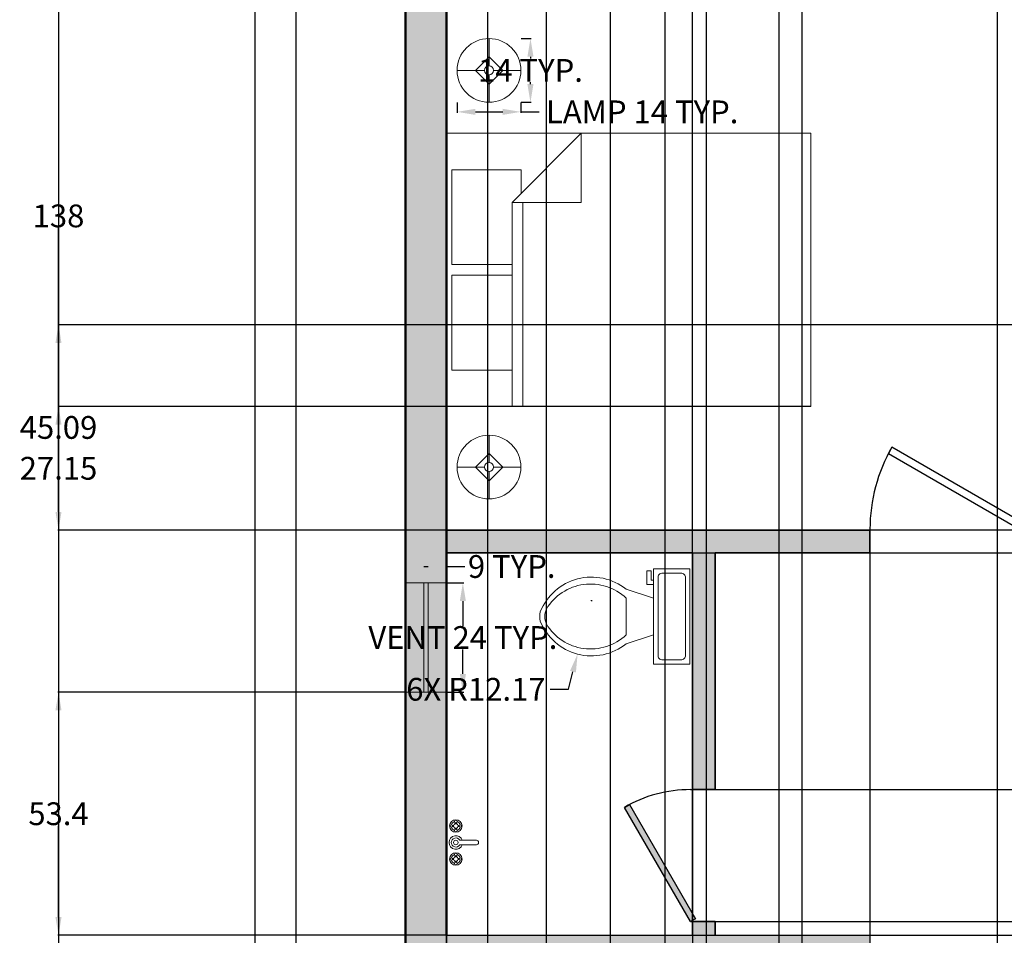
# Model space of a CAD drawing. Units: inches. Extents: x 882 to 1363, y 890 to 1847.
# Tile 7 of 9: x 898 to 1114, y 1479 to 1680. Entities that reach past the tile are written whole.
import ezdxf

# ---------------------------------------------------------------- set-up
doc = ezdxf.new("R2010")
doc.units = ezdxf.units.IN
doc.header["$MEASUREMENT"] = 0
for name, color, linetype, lineweight in [('A-ANNO-DIMS', 2, 'Continuous', 18), ('A-WALL-PATT-BNDY', 7, 'Continuous', 13), ('C-PROP', 7, 'Continuous', 25), ('doors', 3, 'Continuous', 25), ('furniture', 10, 'Continuous', 18), ('inner wall', 50, 'Continuous', 35), ('outer wall', 40, 'Continuous', 50), ('sanitary', 231, 'Continuous', 18), ('ventilator', 130, 'Continuous', 18)]:
    doc.layers.add(name, color=color, linetype=linetype, lineweight=lineweight)
doc.layers.add('A-WALL-PATT', color=251, linetype='Continuous', lineweight=13, true_color=0x636466)
doc.styles.get("Standard").update_dxf_attribs({"font": 'arial.ttf'})
doc.dimstyles.get("Standard").update_dxf_attribs({"dimtxt": 5, "dimasz": 4, "dimexe": 0.18, "dimexo": 0.0625, "dimgap": 0.09, "dimtad": 0, "dimtih": 1, "dimtoh": 1, "dimdec": 1, "dimzin": 0, "dimdsep": 46, "dimlunit": 3, "dimtxsty": 'Standard', "dimcen": 0.09, "dimadec": 0, "dimazin": 0, "dimtfac": 1, "dimtdec": 1, "dimtofl": 0, "dimtmove": 0, "dimatfit": 3, "dimfxl": 1, "dimtolj": 1, "dimtzin": 0, "dimarcsym": 0})

# ---------------------------------------------------------------- blocks, each defined once
blk = doc.blocks.new('*U3')
for p, q in [((0, 0), (0, 6)), ((40, 0), (40, 6))]:
    blk.add_line(p, q)
blk.add_lwpolyline([(0, 0), (34.64, -20), (35.52, -18.48), (0.87, 1.52)], close=True)
blk.add_arc((0, 0), 40, 330, 0)
blk = doc.blocks.new('*U5')
for p, q in [((0, 0), (0, -6)), ((40, 0), (40, -6))]:
    blk.add_line(p, q)
blk.add_lwpolyline([(0, 0), (34.64, 20), (35.52, 18.48), (0.88, -1.52)], close=True)
blk.add_arc((0, 0), 40, 0, 30)
blk = doc.blocks.new('Toilet - top')
for p, q in [((9.5, -6), (9.5, -2)), ((-10, -8.5), (-8, -8.5)), ((-10, -9.5), (-10, -8.5)), ((-8, -8.5), (-8, -8)), ((-7, -8), (-7, -9.5)), ((-4, -8), (-6, -14)), ((4, -8), (6, -14)), ((-7, -9.5), (-10, -9.5)), ((4, -14), (-4, -14))]:
    blk.add_line(p, q)
blk.add_lwpolyline([(10.5, -8), (10.5, 0), (-10.5, 0), (-10.5, -8)], close=True)
for points in [[(-9.5, -2), (-9.5, -6)], [(8.5, -1), (-8.5, -1)], [(-8.5, -7), (8.5, -7)]]:
    blk.add_lwpolyline(points)
for centre, radius, start, end in [((-8.62, -1.88), 0.884, 81.8699, 188.1301), ((8.62, -1.88), 0.884, 351.8699, 98.1301), ((-8.62, -6.12), 0.884, 171.8699, 278.1301), ((8.62, -6.12), 0.884, 261.8699, 8.1301), ((3.52, -21.58), 12.17, 141.4691, 247.9714), ((4.2, -21.82), 11.33, 136.3677, 238.9468), ((-3.52, -21.58), 12.17, 292.0284, 38.5307), ((-4.2, -21.82), 11.33, 301.053, 43.6321), ((0, -27.88), 4, 245.7318, 294.2682), ((0, -29), 4, 254.8605, 285.1395)]:
    blk.add_arc(centre, radius, start, end)
blk = doc.blocks.new('Faucet - Bathroom top')
for p, q in [((-4.107, 0.125), (-4.375, 0.125)), ((-3.75, 0.4788), (-3.75, 0.75)), ((-3.5, 0.482), (-3.5, 0.75)), ((-3.1461, 0.125), (-2.875, 0.125)), ((3.143, 0.125), (2.875, 0.125)), ((3.5, 0.4788), (3.5, 0.75)), ((3.75, 0.482), (3.75, 0.75)), ((4.1039, 0.125), (4.375, 0.125)), ((-4.1039, -0.125), (-4.375, -0.125)), ((-3.75, -0.4821), (-3.75, -0.75)), ((-3.5, -0.4789), (-3.5, -0.75)), ((-3.143, -0.125), (-2.875, -0.125)), ((-0.5, -0.8639), (-0.5, -4.5)), ((0.5, -4.5), (0.5, -0.8631)), ((3.1461, -0.125), (2.875, -0.125)), ((3.5, -0.4821), (3.5, -0.75)), ((3.75, -0.4789), (3.75, -0.75)), ((4.107, -0.125), (4.375, -0.125))]:
    blk.add_line(p, q)
for centre, radius in [((-3.625, 0), 1.375), ((-4.625, 0), 0.2795), ((-3.625, 0), 0.5), ((-3.625, 1), 0.2795), ((-2.625, 0), 0.2795), ((0, 0), 0.5), ((3.625, 0), 1.375), ((2.625, 0), 0.2795), ((3.625, 0), 0.5), ((3.625, 1), 0.2795), ((4.625, 0), 0.2795), ((-3.625, -1), 0.2795), ((3.625, -1), 0.2795)]:
    blk.add_circle(centre, radius)
for centre, radius, start, end in [((-3.625, 0), 1, 105.2407, 164.2093), ((-3.625, 0), 1, 16.44125, 74.07887), ((0, 0), 1.5, 289.6514, 250.3603), ((0, 0), 1, 300.3431, 239.7554), ((3.625, 0), 1, 106.12, 164.0884), ((3.625, 0), 1, 16.23422, 73.90469), ((-3.625, 0), 1, 196.2342, 253.9047), ((-3.625, 0), 1, 286.12, 344.0884), ((3.625, 0), 1, 196.4413, 254.0789), ((3.625, 0), 1, 285.2407, 344.2093), ((0, -4.5), 0.5, 180, 0)]:
    blk.add_arc(centre, radius, start, end)
blk = doc.blocks.new('Bed - Queen')
for p, q in [((0, -80.00003), (0, 0)), ((0, 0), (59.99999, 0)), ((59.99999, 0), (59.99999, -80.00003)), ((7.99999, -1.2), (28.79998, -1.2)), ((7.99999, -14.4), (7.99999, -1.2)), ((28.79998, -1.2), (28.79998, -14.4)), ((31.19999, -1.2), (51.99999, -1.2)), ((31.19999, -14.4), (31.19999, -1.2)), ((51.99999, -1.2), (51.99999, -16.4)), ((0, -14.4), (44.8, -14.4)), ((59.99999, -29.6), (44.8, -14.4)), ((44.8, -14.4), (44.8, -29.6)), ((44.8, -16.8), (0, -16.8)), ((51.99999, -16.4), (46.79936, -16.4)), ((44.8, -29.6), (59.99999, -29.6)), ((59.99999, -80.00003), (0, -80.00003))]:
    blk.add_line(p, q)
blk = doc.blocks.new('Lamp - Table')
for p, q in [((0, 7), (0, 1)), ((0, 3), (-3, 0)), ((3, 0), (0, 3)), ((-1, 0), (-7, 0)), ((-3, 0), (0, -3)), ((0, -3), (3, 0)), ((1, 0), (7, 0)), ((0, -1), (0, -7))]:
    blk.add_line(p, q)
for radius in [7, 1]:
    blk.add_circle((0, 0), radius)
blk = doc.blocks.new('VENT-24IN-9IN')
for p, q in [((24, 5), (0, 5)), ((24, 4), (0, 4))]:
    blk.add_line(p, q)
blk.add_lwpolyline([(0, 9), (24, 9), (24, 0), (0, 0)], close=True)
blk = doc.blocks.new('*D17')
at = {"layer": 'A-ANNO-DIMS', "color": 0, "lineweight": -2, "transparency": 16777216}
for p, q in [((994.18, 1661.64), (994.18, 1659.42)), ((1008.18, 1661.64), (1008.18, 1659.42)), ((998.18, 1659.6), (1004.18, 1659.6)), ((1008.18, 1659.6), (1012.18, 1659.6))]:
    blk.add_line(p, q, dxfattribs=at)
at = {"layer": 'A-ANNO-DIMS', "color": 0, "transparency": 16777216}
for points in [[(998.18, 1660.27), (998.18, 1658.93), (994.18, 1659.6)], [(1004.18, 1660.27), (1004.18, 1658.93), (1008.18, 1659.6)]]:
    blk.add_solid(points, dxfattribs=at)
at = {"layer": 'Defpoints', "color": 0, "transparency": 16777216}
for p in [(994.18, 1661.7), (1008.18, 1661.7), (1008.18, 1659.6)]:
    blk.add_point(p, dxfattribs=at)
at = {"layer": 'A-ANNO-DIMS', "color": 0, "transparency": 16777216, "insert": (1034.81, 1659.6), "char_height": 5, "attachment_point": 5}
blk.add_mtext('\\A1;LAMP 14 TYP.', dxfattribs=at)
blk = doc.blocks.new('*D18')
at = {"layer": 'A-ANNO-DIMS', "color": 0, "lineweight": -2, "transparency": 16777216}
for p, q in [((1008.24, 1675.7), (1010.46, 1675.7)), ((1010.28, 1671.7), (1010.28, 1671.3)), ((1010.28, 1665.7), (1010.28, 1666.1)), ((1008.24, 1661.7), (1010.46, 1661.7))]:
    blk.add_line(p, q, dxfattribs=at)
at = {"layer": 'A-ANNO-DIMS', "color": 0, "transparency": 16777216}
for points in [[(1009.61, 1671.7), (1010.95, 1671.7), (1010.28, 1675.7)], [(1009.61, 1665.7), (1010.95, 1665.7), (1010.28, 1661.7)]]:
    blk.add_solid(points, dxfattribs=at)
at = {"layer": 'Defpoints', "color": 0, "transparency": 16777216}
for p in [(1008.18, 1675.7), (1010.28, 1675.7), (1008.18, 1661.7)]:
    blk.add_point(p, dxfattribs=at)
at = {"layer": 'A-ANNO-DIMS', "color": 0, "transparency": 16777216, "insert": (1010.28, 1668.7), "char_height": 5, "attachment_point": 5}
blk.add_mtext('\\A1;14 TYP.', dxfattribs=at)
blk = doc.blocks.new('*D25')
at = {"layer": 'A-ANNO-DIMS', "color": 0, "lineweight": -2, "transparency": 16777216}
for p, q in [((991.9, 1556.15), (995.62, 1556.15)), ((995.44, 1552.15), (995.44, 1546.75)), ((995.44, 1536.15), (995.44, 1541.55)), ((991.9, 1532.15), (995.62, 1532.15))]:
    blk.add_line(p, q, dxfattribs=at)
at = {"layer": 'A-ANNO-DIMS', "color": 0, "transparency": 16777216}
for points in [[(994.77, 1552.15), (996.11, 1552.15), (995.44, 1556.15)], [(994.77, 1536.15), (996.11, 1536.15), (995.44, 1532.15)]]:
    blk.add_solid(points, dxfattribs=at)
at = {"layer": 'Defpoints', "color": 0, "transparency": 16777216}
for p in [(991.84, 1556.15), (991.84, 1532.15), (995.44, 1532.15)]:
    blk.add_point(p, dxfattribs=at)
at = {"layer": 'A-ANNO-DIMS', "color": 0, "transparency": 16777216, "insert": (995.44, 1544.15), "char_height": 5, "attachment_point": 5}
blk.add_mtext('\\A1;VENT 24 TYP.', dxfattribs=at)
blk = doc.blocks.new('*D26')
at = {"layer": 'A-ANNO-DIMS', "color": 0, "lineweight": -2, "transparency": 16777216}
for p, q in [((982.84, 1556.22), (982.84, 1559.93)), ((986.84, 1559.75), (987.84, 1559.75)), ((991.84, 1556.22), (991.84, 1559.93)), ((991.84, 1559.75), (995.84, 1559.75))]:
    blk.add_line(p, q, dxfattribs=at)
at = {"layer": 'A-ANNO-DIMS', "color": 0, "transparency": 16777216}
for points in [[(986.84, 1560.42), (986.84, 1559.09), (982.84, 1559.75)], [(987.84, 1560.42), (987.84, 1559.09), (991.84, 1559.75)]]:
    blk.add_solid(points, dxfattribs=at)
at = {"layer": 'Defpoints', "color": 0, "transparency": 16777216}
for p in [(991.84, 1559.75), (982.84, 1556.15), (991.84, 1556.15)]:
    blk.add_point(p, dxfattribs=at)
at = {"layer": 'A-ANNO-DIMS', "color": 0, "transparency": 16777216, "insert": (1006.16, 1559.75), "char_height": 5, "attachment_point": 5}
blk.add_mtext('\\A1;9 TYP.', dxfattribs=at)
blk = doc.blocks.new('*D37')
at = {"layer": 'A-ANNO-DIMS', "color": 0, "lineweight": -2, "transparency": 16777216}
for p, q in [((982.78, 1767.75), (906.46, 1767.75)), ((906.64, 1763.75), (906.64, 1383.34)), ((906.64, 997.75), (906.64, 1378.16)), ((982.78, 993.75), (906.46, 993.75))]:
    blk.add_line(p, q, dxfattribs=at)
at = {"layer": 'A-ANNO-DIMS', "color": 0, "transparency": 16777216}
for points in [[(905.97, 1763.75), (907.3, 1763.75), (906.64, 1767.75)], [(905.97, 997.75), (907.3, 997.75), (906.64, 993.75)]]:
    blk.add_solid(points, dxfattribs=at)
at = {"layer": 'Defpoints', "color": 0, "transparency": 16777216}
for p in [(906.64, 1767.75), (982.84, 1767.75), (982.84, 993.75)]:
    blk.add_point(p, dxfattribs=at)
at = {"layer": 'A-ANNO-DIMS', "color": 0, "transparency": 16777216, "insert": (906.64, 1380.75), "char_height": 5, "attachment_point": 5}
blk.add_mtext('\\A1;774', dxfattribs=at)
blk = doc.blocks.new('*D40')
at = {"layer": 'A-ANNO-DIMS', "color": 0, "lineweight": -2, "transparency": 16777216}
for p, q in [((991.84, 1758.69), (991.84, 893.37)), ((1064.84, 1758.69), (1064.84, 893.37)), ((995.84, 893.55), (1024.69, 893.55)), ((1060.84, 893.55), (1031.99, 893.55))]:
    blk.add_line(p, q, dxfattribs=at)
at = {"layer": 'A-ANNO-DIMS', "color": 0, "transparency": 16777216}
for points in [[(995.84, 894.21), (995.84, 892.88), (991.84, 893.55)], [(1060.84, 894.21), (1060.84, 892.88), (1064.84, 893.55)]]:
    blk.add_solid(points, dxfattribs=at)
at = {"layer": 'Defpoints', "color": 0, "transparency": 16777216}
for p in [(991.84, 1758.75), (1064.84, 1758.75), (1064.84, 893.55)]:
    blk.add_point(p, dxfattribs=at)
at = {"layer": 'A-ANNO-DIMS', "color": 0, "transparency": 16777216, "insert": (1028.34, 893.55), "char_height": 5, "attachment_point": 5}
blk.add_mtext('\\A1;73', dxfattribs=at)
blk = doc.blocks.new('*D41')
at = {"layer": 'A-ANNO-DIMS', "color": 0, "lineweight": -2, "transparency": 16777216}
for p, q in [((1069.84, 1758.69), (1069.84, 893.37)), ((1154.84, 1758.69), (1154.84, 893.37)), ((1073.84, 893.55), (1108.65, 893.55)), ((1150.84, 893.55), (1116.03, 893.55))]:
    blk.add_line(p, q, dxfattribs=at)
at = {"layer": 'A-ANNO-DIMS', "color": 0, "transparency": 16777216}
for points in [[(1073.84, 894.21), (1073.84, 892.88), (1069.84, 893.55)], [(1150.84, 894.21), (1150.84, 892.88), (1154.84, 893.55)]]:
    blk.add_solid(points, dxfattribs=at)
at = {"layer": 'Defpoints', "color": 0, "transparency": 16777216}
for p in [(1069.84, 1758.75), (1154.84, 1758.75), (1154.84, 893.55)]:
    blk.add_point(p, dxfattribs=at)
at = {"layer": 'A-ANNO-DIMS', "color": 0, "transparency": 16777216, "insert": (1112.34, 893.55), "char_height": 5, "attachment_point": 5}
blk.add_mtext('\\A1;85', dxfattribs=at)
blk = doc.blocks.new('*D44')
at = {"layer": 'A-ANNO-DIMS', "color": 0, "lineweight": -2, "transparency": 16777216}
for p, q in [((1243.78, 1705.75), (906.46, 1705.75)), ((906.64, 1701.75), (906.64, 1639.39)), ((906.64, 1571.75), (906.64, 1634.1)), ((1243.78, 1567.75), (906.46, 1567.75))]:
    blk.add_line(p, q, dxfattribs=at)
at = {"layer": 'A-ANNO-DIMS', "color": 0, "transparency": 16777216}
for points in [[(905.97, 1701.75), (907.3, 1701.75), (906.64, 1705.75)], [(905.97, 1571.75), (907.3, 1571.75), (906.64, 1567.75)]]:
    blk.add_solid(points, dxfattribs=at)
at = {"layer": 'Defpoints', "color": 0, "transparency": 16777216}
for p in [(1243.84, 1705.75), (906.64, 1567.75), (1243.84, 1567.75)]:
    blk.add_point(p, dxfattribs=at)
at = {"layer": 'A-ANNO-DIMS', "color": 0, "transparency": 16777216, "insert": (906.64, 1636.75), "char_height": 5, "attachment_point": 5}
blk.add_mtext('\\A1;138', dxfattribs=at)
blk = doc.blocks.new('*D46')
at = {"layer": 'A-ANNO-DIMS', "color": 0, "lineweight": -2, "transparency": 16777216}
for p, q in [((991.84, 1567.81), (991.84, 1844.13)), ((995.84, 1843.95), (1052.49, 1843.95)), ((1119.84, 1843.95), (1063.19, 1843.95)), ((1123.84, 1567.81), (1123.84, 1844.13))]:
    blk.add_line(p, q, dxfattribs=at)
at = {"layer": 'A-ANNO-DIMS', "color": 0, "transparency": 16777216}
for points in [[(995.84, 1844.62), (995.84, 1843.29), (991.84, 1843.95)], [(1119.84, 1844.62), (1119.84, 1843.29), (1123.84, 1843.95)]]:
    blk.add_solid(points, dxfattribs=at)
at = {"layer": 'Defpoints', "color": 0, "transparency": 16777216}
for p in [(1123.84, 1843.95), (991.84, 1567.75), (1123.84, 1567.75)]:
    blk.add_point(p, dxfattribs=at)
at = {"layer": 'A-ANNO-DIMS', "color": 0, "transparency": 16777216, "insert": (1057.84, 1843.95), "char_height": 5, "attachment_point": 5}
blk.add_mtext('\\A1;132', dxfattribs=at)
blk = doc.blocks.new('*D48')
at = {"layer": 'A-ANNO-DIMS', "color": 0, "lineweight": -2, "transparency": 16777216}
for p, q in [((1084.84, 1562.69), (1084.84, 893.37)), ((1120.84, 1562.69), (1120.84, 893.37)), ((1088.84, 893.55), (1099.17, 893.55)), ((1116.84, 893.55), (1106.51, 893.55))]:
    blk.add_line(p, q, dxfattribs=at)
at = {"layer": 'A-ANNO-DIMS', "color": 0, "transparency": 16777216}
for points in [[(1088.84, 894.21), (1088.84, 892.88), (1084.84, 893.55)], [(1116.84, 894.21), (1116.84, 892.88), (1120.84, 893.55)]]:
    blk.add_solid(points, dxfattribs=at)
at = {"layer": 'Defpoints', "color": 0, "transparency": 16777216}
for p in [(1084.84, 1562.75), (1120.84, 1562.75), (1120.84, 893.55)]:
    blk.add_point(p, dxfattribs=at)
at = {"layer": 'A-ANNO-DIMS', "color": 0, "transparency": 16777216, "insert": (1102.84, 893.55), "char_height": 5, "attachment_point": 5}
blk.add_mtext('\\A1;36', dxfattribs=at)
blk = doc.blocks.new('*D51')
at = {"layer": 'A-ANNO-DIMS', "color": 0, "lineweight": -2, "transparency": 16777216}
for p, q in [((982.84, 1767.69), (982.84, 893.37)), ((1000.84, 1767.69), (1000.84, 893.37)), ((986.84, 893.55), (996.84, 893.55)), ((1000.84, 893.55), (1004.84, 893.55))]:
    blk.add_line(p, q, dxfattribs=at)
at = {"layer": 'A-ANNO-DIMS', "color": 0, "transparency": 16777216}
for points in [[(986.84, 894.21), (986.84, 892.88), (982.84, 893.55)], [(996.84, 894.21), (996.84, 892.88), (1000.84, 893.55)]]:
    blk.add_solid(points, dxfattribs=at)
at = {"layer": 'Defpoints', "color": 0, "transparency": 16777216}
for p in [(982.84, 1767.75), (1000.84, 1767.75), (1000.84, 893.55)]:
    blk.add_point(p, dxfattribs=at)
at = {"layer": 'A-ANNO-DIMS', "color": 0, "transparency": 16777216, "insert": (1015.08, 893.55), "char_height": 5, "attachment_point": 5}
blk.add_mtext('\\A1;18.006', dxfattribs=at)
blk = doc.blocks.new('*D52')
at = {"layer": 'A-ANNO-DIMS', "color": 0, "lineweight": -2, "transparency": 16777216}
for p, q in [((1048.84, 1767.69), (1048.84, 893.37)), ((1118.86, 1767.69), (1118.86, 893.37)), ((1052.84, 893.55), (1075.83, 893.55)), ((1114.86, 893.55), (1091.87, 893.55))]:
    blk.add_line(p, q, dxfattribs=at)
at = {"layer": 'A-ANNO-DIMS', "color": 0, "transparency": 16777216}
for points in [[(1052.84, 894.21), (1052.84, 892.88), (1048.84, 893.55)], [(1114.86, 894.21), (1114.86, 892.88), (1118.86, 893.55)]]:
    blk.add_solid(points, dxfattribs=at)
at = {"layer": 'Defpoints', "color": 0, "transparency": 16777216}
for p in [(1048.84, 1767.75), (1118.86, 1767.75), (1118.86, 893.55)]:
    blk.add_point(p, dxfattribs=at)
at = {"layer": 'A-ANNO-DIMS', "color": 0, "transparency": 16777216, "insert": (1083.85, 893.55), "char_height": 5, "attachment_point": 5}
blk.add_mtext('\\A1;70.01', dxfattribs=at)
blk = doc.blocks.new('*D56')
at = {"layer": 'A-ANNO-DIMS', "color": 0, "lineweight": -2, "transparency": 16777216}
for p, q in [((991.9, 1562.75), (1353.22, 1562.75)), ((1353.04, 1558.75), (1353.04, 1523.39)), ((1353.04, 1482.75), (1353.04, 1518.11)), ((991.9, 1478.75), (1353.22, 1478.75))]:
    blk.add_line(p, q, dxfattribs=at)
at = {"layer": 'A-ANNO-DIMS', "color": 0, "transparency": 16777216}
for points in [[(1352.38, 1558.75), (1353.71, 1558.75), (1353.04, 1562.75)], [(1352.38, 1482.75), (1353.71, 1482.75), (1353.04, 1478.75)]]:
    blk.add_solid(points, dxfattribs=at)
at = {"layer": 'Defpoints', "color": 0, "transparency": 16777216}
for p in [(991.84, 1562.75), (991.84, 1478.75), (1353.04, 1478.75)]:
    blk.add_point(p, dxfattribs=at)
at = {"layer": 'A-ANNO-DIMS', "color": 0, "transparency": 16777216, "insert": (1353.04, 1520.75), "char_height": 5, "attachment_point": 5}
blk.add_mtext('\\A1;84', dxfattribs=at)
blk = doc.blocks.new('*D57')
at = {"layer": 'A-ANNO-DIMS', "color": 0, "lineweight": -2, "transparency": 16777216}
for p, q in [((991.84, 1478.81), (991.84, 1844.13)), ((995.84, 1843.95), (1015.18, 1843.95)), ((1041.84, 1843.95), (1022.5, 1843.95)), ((1045.84, 1478.81), (1045.84, 1844.13))]:
    blk.add_line(p, q, dxfattribs=at)
at = {"layer": 'A-ANNO-DIMS', "color": 0, "transparency": 16777216}
for points in [[(995.84, 1844.62), (995.84, 1843.29), (991.84, 1843.95)], [(1041.84, 1844.62), (1041.84, 1843.29), (1045.84, 1843.95)]]:
    blk.add_solid(points, dxfattribs=at)
at = {"layer": 'Defpoints', "color": 0, "transparency": 16777216}
for p in [(1045.84, 1843.95), (991.84, 1478.75), (1045.84, 1478.75)]:
    blk.add_point(p, dxfattribs=at)
at = {"layer": 'A-ANNO-DIMS', "color": 0, "transparency": 16777216, "insert": (1018.84, 1843.95), "char_height": 5, "attachment_point": 5}
blk.add_mtext('\\A1;54', dxfattribs=at)
blk = doc.blocks.new('*D60')
at = {"layer": 'A-ANNO-DIMS', "color": 0, "lineweight": -2, "transparency": 16777216}
for p, q in [((1050.9, 1510.75), (1353.22, 1510.75)), ((1353.04, 1506.75), (1353.04, 1498.89)), ((1353.04, 1485.75), (1353.04, 1493.61)), ((1050.9, 1481.75), (1353.22, 1481.75))]:
    blk.add_line(p, q, dxfattribs=at)
at = {"layer": 'A-ANNO-DIMS', "color": 0, "transparency": 16777216}
for points in [[(1352.38, 1506.75), (1353.71, 1506.75), (1353.04, 1510.75)], [(1352.38, 1485.75), (1353.71, 1485.75), (1353.04, 1481.75)]]:
    blk.add_solid(points, dxfattribs=at)
at = {"layer": 'Defpoints', "color": 0, "transparency": 16777216}
for p in [(1050.84, 1510.75), (1050.84, 1481.75), (1353.04, 1481.75)]:
    blk.add_point(p, dxfattribs=at)
at = {"layer": 'A-ANNO-DIMS', "color": 0, "transparency": 16777216, "insert": (1353.04, 1496.25), "char_height": 5, "attachment_point": 5}
blk.add_mtext('\\A1;29', dxfattribs=at)
blk = doc.blocks.new('*D68')
at = {"layer": 'A-ANNO-DIMS', "color": 0, "lineweight": -2, "transparency": 16777216}
for p, q in [((1027.84, 1142.81), (1027.84, 1844.13)), ((1031.84, 1843.95), (1066.65, 1843.95)), ((1108.84, 1843.95), (1074.03, 1843.95)), ((1112.84, 1142.81), (1112.84, 1844.13))]:
    blk.add_line(p, q, dxfattribs=at)
at = {"layer": 'A-ANNO-DIMS', "color": 0, "transparency": 16777216}
for points in [[(1031.84, 1844.62), (1031.84, 1843.29), (1027.84, 1843.95)], [(1108.84, 1844.62), (1108.84, 1843.29), (1112.84, 1843.95)]]:
    blk.add_solid(points, dxfattribs=at)
at = {"layer": 'Defpoints', "color": 0, "transparency": 16777216}
for p in [(1112.84, 1843.95), (1027.84, 1142.75), (1112.84, 1142.75)]:
    blk.add_point(p, dxfattribs=at)
at = {"layer": 'A-ANNO-DIMS', "color": 0, "transparency": 16777216, "insert": (1070.34, 1843.95), "char_height": 5, "attachment_point": 5}
blk.add_mtext('\\A1;85', dxfattribs=at)
blk = doc.blocks.new('*D74')
at = {"layer": 'A-ANNO-DIMS', "color": 0, "lineweight": -2, "transparency": 16777216}
for p, q in [((991.84, 1002.81), (991.84, 1844.13)), ((995.84, 1843.95), (1012.06, 1843.95)), ((1035.84, 1843.95), (1019.62, 1843.95)), ((1039.84, 1002.81), (1039.84, 1844.13))]:
    blk.add_line(p, q, dxfattribs=at)
at = {"layer": 'A-ANNO-DIMS', "color": 0, "transparency": 16777216}
for points in [[(995.84, 1844.62), (995.84, 1843.29), (991.84, 1843.95)], [(1035.84, 1844.62), (1035.84, 1843.29), (1039.84, 1843.95)]]:
    blk.add_solid(points, dxfattribs=at)
at = {"layer": 'Defpoints', "color": 0, "transparency": 16777216}
for p in [(1039.84, 1843.95), (991.84, 1002.75), (1039.84, 1002.75)]:
    blk.add_point(p, dxfattribs=at)
at = {"layer": 'A-ANNO-DIMS', "color": 0, "transparency": 16777216, "insert": (1015.84, 1843.95), "char_height": 5, "attachment_point": 5}
blk.add_mtext('\\A1;48', dxfattribs=at)
blk = doc.blocks.new('*D85')
at = {"layer": 'A-ANNO-DIMS', "color": 0, "lineweight": -2, "transparency": 16777216}
for p, q in [((1045.84, 1562.69), (1045.84, 893.37)), ((1084.84, 1562.69), (1084.84, 893.37)), ((1049.84, 893.55), (1061.66, 893.55)), ((1080.84, 893.55), (1069.01, 893.55))]:
    blk.add_line(p, q, dxfattribs=at)
at = {"layer": 'A-ANNO-DIMS', "color": 0, "transparency": 16777216}
for points in [[(1049.84, 894.21), (1049.84, 892.88), (1045.84, 893.55)], [(1080.84, 894.21), (1080.84, 892.88), (1084.84, 893.55)]]:
    blk.add_solid(points, dxfattribs=at)
at = {"layer": 'Defpoints', "color": 0, "transparency": 16777216}
for p in [(1045.84, 1562.75), (1084.84, 1562.75), (1084.84, 893.55)]:
    blk.add_point(p, dxfattribs=at)
at = {"layer": 'A-ANNO-DIMS', "color": 0, "transparency": 16777216, "insert": (1065.34, 893.55), "char_height": 5, "attachment_point": 5}
blk.add_mtext('\\A1;39', dxfattribs=at)
blk = doc.blocks.new('*D87')
at = {"layer": 'A-ANNO-DIMS', "color": 0, "lineweight": -2, "transparency": 16777216}
for p, q in [((982.78, 1532.15), (906.46, 1532.15)), ((906.64, 1528.15), (906.64, 1508.1)), ((906.64, 1482.75), (906.64, 1502.81)), ((991.78, 1478.75), (906.46, 1478.75))]:
    blk.add_line(p, q, dxfattribs=at)
at = {"layer": 'A-ANNO-DIMS', "color": 0, "transparency": 16777216}
for points in [[(905.97, 1528.15), (907.3, 1528.15), (906.64, 1532.15)], [(905.97, 1482.75), (907.3, 1482.75), (906.64, 1478.75)]]:
    blk.add_solid(points, dxfattribs=at)
at = {"layer": 'Defpoints', "color": 0, "transparency": 16777216}
for p in [(982.84, 1532.15), (906.64, 1478.75), (991.84, 1478.75)]:
    blk.add_point(p, dxfattribs=at)
at = {"layer": 'A-ANNO-DIMS', "color": 0, "transparency": 16777216, "insert": (906.64, 1505.45), "char_height": 5, "attachment_point": 5}
blk.add_mtext('\\A1;53.4', dxfattribs=at)
blk = doc.blocks.new('*D90')
at = {"layer": 'A-ANNO-DIMS', "color": 0, "lineweight": -2, "transparency": 16777216}
for p, q in [((1071.78, 1594.9), (906.46, 1594.9)), ((906.64, 1590.9), (906.64, 1583.97)), ((906.64, 1571.75), (906.64, 1578.68)), ((1084.78, 1567.75), (906.46, 1567.75))]:
    blk.add_line(p, q, dxfattribs=at)
at = {"layer": 'A-ANNO-DIMS', "color": 0, "transparency": 16777216}
for points in [[(905.97, 1590.9), (907.3, 1590.9), (906.64, 1594.9)], [(905.97, 1571.75), (907.3, 1571.75), (906.64, 1567.75)]]:
    blk.add_solid(points, dxfattribs=at)
at = {"layer": 'Defpoints', "color": 0, "transparency": 16777216}
for p in [(1071.84, 1594.9), (906.64, 1567.75), (1084.84, 1567.75)]:
    blk.add_point(p, dxfattribs=at)
at = {"layer": 'A-ANNO-DIMS', "color": 0, "transparency": 16777216, "insert": (906.64, 1581.32), "char_height": 5, "attachment_point": 5}
blk.add_mtext('\\A1;27.15', dxfattribs=at)
blk = doc.blocks.new('*D91')
at = {"layer": 'A-ANNO-DIMS', "color": 0, "lineweight": -2, "transparency": 16777216}
for p, q in [((1208.78, 1612.84), (906.46, 1612.84)), ((906.64, 1608.84), (906.64, 1592.94)), ((906.64, 1571.75), (906.64, 1587.65)), ((1211.78, 1567.75), (906.46, 1567.75))]:
    blk.add_line(p, q, dxfattribs=at)
at = {"layer": 'A-ANNO-DIMS', "color": 0, "transparency": 16777216}
for points in [[(905.97, 1608.84), (907.3, 1608.84), (906.64, 1612.84)], [(905.97, 1571.75), (907.3, 1571.75), (906.64, 1567.75)]]:
    blk.add_solid(points, dxfattribs=at)
at = {"layer": 'Defpoints', "color": 0, "transparency": 16777216}
for p in [(1208.84, 1612.84), (906.64, 1567.75), (1211.84, 1567.75)]:
    blk.add_point(p, dxfattribs=at)
at = {"layer": 'A-ANNO-DIMS', "color": 0, "transparency": 16777216, "insert": (906.64, 1590.29), "char_height": 5, "attachment_point": 5}
blk.add_mtext('\\A1;45.09', dxfattribs=at)
blk = doc.blocks.new('*D93')
at = {"layer": 'A-ANNO-DIMS', "color": 0, "lineweight": -2, "transparency": 16777216}
for p, q in [((987.84, 1843.95), (983.84, 1843.95)), ((991.84, 1337.4), (991.84, 1844.13)), ((1013.79, 1306.45), (1013.79, 1844.13)), ((1017.79, 1843.95), (1021.79, 1843.95))]:
    blk.add_line(p, q, dxfattribs=at)
at = {"layer": 'A-ANNO-DIMS', "color": 0, "transparency": 16777216}
for points in [[(987.84, 1844.62), (987.84, 1843.29), (991.84, 1843.95)], [(1017.79, 1844.62), (1017.79, 1843.29), (1013.79, 1843.95)]]:
    blk.add_solid(points, dxfattribs=at)
at = {"layer": 'Defpoints', "color": 0, "transparency": 16777216}
for p in [(1013.79, 1843.95), (991.84, 1337.33), (1013.79, 1306.39)]:
    blk.add_point(p, dxfattribs=at)
at = {"layer": 'A-ANNO-DIMS', "color": 0, "transparency": 16777216, "insert": (1002.81, 1843.95), "char_height": 5, "attachment_point": 5}
blk.add_mtext('\\A1;21.95', dxfattribs=at)
blk = doc.blocks.new('*D95')
at = {"layer": 'A-ANNO-DIMS', "color": 0, "lineweight": -2, "transparency": 16777216}
for p, q in [((1023.63, 1552.29), (1023.81, 1552.29)), ((1023.72, 1552.2), (1023.72, 1552.38)), ((1018.6, 1532.78), (1019.62, 1536.65)), ((1014.6, 1532.78), (1018.6, 1532.78))]:
    blk.add_line(p, q, dxfattribs=at)
at = {"layer": 'A-ANNO-DIMS', "color": 0, "transparency": 16777216}
blk.add_solid([(1018.97, 1536.82), (1020.26, 1536.48), (1020.63, 1540.52)], dxfattribs=at)
at = {"layer": 'Defpoints', "color": 0, "transparency": 16777216}
for p in [(1023.72, 1552.29), (1020.63, 1540.52)]:
    blk.add_point(p, dxfattribs=at)
at = {"layer": 'A-ANNO-DIMS', "color": 0, "transparency": 16777216, "insert": (998.3, 1532.78), "char_height": 5, "attachment_point": 5}
blk.add_mtext('\\A1;6X R12.17', dxfattribs=at)

msp = doc.modelspace()

# ---------------------------------------------------------------- hatches: boundary and pattern name
at = {"layer": 'A-WALL-PATT'}
h = msp.add_hatch(color=256, dxfattribs=at)
h.dxf.hatch_style = 1
h.paths.add_polyline_path([(1050.8388, 1481.7495), (1050.8388, 1478.7495), (1084.8388, 1478.7495), (1084.8388, 1473.7495), (991.8388, 1473.7495), (991.8388, 1361.0778), (982.8388, 1361.0778), (982.8388, 1556.1531), (991.8388, 1556.1531), (991.8388, 1478.7495), (1045.8388, 1478.7495), (1045.8388, 1481.7479), (1045.4161, 1481.7477), (1030.9055, 1506.8563), (1032.004, 1507.4911), (1046.5146, 1482.3825), (1045.4161, 1481.7477), (1045.8388, 1481.7479), (1045.8388, 1481.7495)])
h.paths.add_polyline_path([(1128.8388, 1478.7495), (1120.8388, 1478.7495), (1120.8388, 1473.7495), (1123.8388, 1473.7495), (1123.8388, 1353.7495), (991.8388, 1353.7495), (991.8388, 1361.0778), (982.8388, 1361.0778), (982.8388, 1337.3333), (991.8388, 1337.3333), (991.8388, 1348.7495), (1128.8388, 1348.7495)])
h.paths.add_polyline_path([(1118.8585, 1767.7495), (1048.8447, 1767.7495), (1048.8447, 1758.7495), (1064.8388, 1758.7495), (1069.8388, 1758.7495), (1118.8585, 1758.7495)])
h.paths.add_polyline_path([(1171.4129, 1767.7495), (1142.8585, 1767.7495), (1142.8585, 1758.7495), (1154.8388, 1758.7495), (1154.8388, 1710.7495), (1069.8388, 1710.7495), (1069.8388, 1713.7495), (1064.8388, 1713.7495), (1064.8388, 1705.7495), (1123.8388, 1705.7495), (1123.8388, 1567.7495), (1120.8388, 1567.7495), (1120.8388, 1562.7495), (1123.8388, 1562.7495), (1211.8388, 1562.7495), (1211.8388, 1567.7495), (1128.8388, 1567.7495), (1128.8388, 1705.7495), (1211.8388, 1705.7495), (1211.8388, 1710.7495), (1159.8388, 1710.7495), (1159.8388, 1758.7495), (1171.4129, 1758.7495)])
h.paths.add_polyline_path([(1252.8388, 1767.7495), (1195.4129, 1767.7495), (1195.4129, 1758.7495), (1243.8388, 1758.7495), (1243.8388, 1710.7495), (1240.8388, 1710.7495), (1240.8388, 1706.4648), (1240.8388, 1705.7495), (1243.8388, 1705.7495), (1243.8388, 1673.1735), (1252.8388, 1673.1735)])
h.paths.add_polyline_path([(1252.8388, 1625.1735), (1243.8388, 1625.1735), (1243.8388, 1567.7495), (1240.8388, 1567.7495), (1240.8388, 1562.7495), (1243.8388, 1562.7495), (1243.8388, 1546.029), (1252.8388, 1546.029)])
h.paths.add_polyline_path([(1252.8388, 1498.029), (1243.8388, 1498.029), (1243.8388, 1391.1399), (1252.8388, 1391.1399)])
h.paths.add_polyline_path([(1252.8388, 1179.8561), (1243.8388, 1179.8561), (1243.8388, 1149.7495), (1219.8388, 1149.7495), (1219.8388, 1145.3111), (1219.8388, 1144.7495), (1252.8388, 1144.7495)])
h.paths.add_polyline_path([(1252.8388, 1277.7495), (1243.8388, 1277.7495), (1243.8388, 1274.7495), (1219.8388, 1274.7495), (1219.8388, 1269.7495), (1243.8388, 1269.7495), (1243.8388, 1227.8561), (1252.8388, 1227.8561)])
h.paths.add_polyline_path([(1252.8388, 1343.1399), (1243.8388, 1343.1399), (1243.8388, 1313.7495), (1248.3388, 1313.7495), (1252.8388, 1313.7495)])
h.paths.add_polyline_path([(1146.8388, 1274.7495), (1112.8388, 1274.7495), (1112.8388, 1106.7495), (1106.7761, 1106.7495), (1106.7761, 1101.7495), (1117.8388, 1101.7495), (1117.8388, 1144.7495), (1159.8388, 1144.7495), (1159.8388, 1149.7495), (1117.8388, 1149.7495), (1117.8388, 1269.7495), (1146.8388, 1269.7495)])
h = msp.add_hatch(color=256, dxfattribs=at)
h.dxf.hatch_style = 1
h.paths.add_polyline_path([(1000.8447, 1767.7495), (993.3979, 1767.7495), (991.8388, 1758.7495), (1000.8447, 1758.7495)])
h.paths.add_polyline_path([(991.8388, 1654.8981), (982.8388, 1654.3544), (982.8388, 1595.0521), (991.8388, 1594.8981)])
h.paths.add_polyline_path([(991.8388, 1594.8981), (982.8388, 1595.0521), (982.8388, 1559.7196), (991.8388, 1562.7495), (991.8388, 1567.7495)])
h.paths.add_polyline_path([(991.8388, 1562.7495), (982.8388, 1559.7196), (982.8388, 1556.1531), (991.8388, 1556.1531)])
h.paths.add_polyline_path([(991.8388, 1289.3333), (982.8388, 1289.3333), (982.8388, 1265.8272), (991.8388, 1265.8272)])
h.paths.add_polyline_path([(1058.7761, 1106.7495), (991.8388, 1106.7495), (982.8388, 1107.8066), (982.8388, 1101.3439), (991.8388, 1101.7495), (1058.7761, 1101.7495)])
h = msp.add_hatch(color=256, dxfattribs=at)
h.dxf.hatch_style = 1
h.paths.add_polyline_path([(993.3979, 1767.7495), (982.8388, 1767.7495), (982.8388, 1752.9363), (991.8388, 1758.7495)])
h.paths.add_polyline_path([(991.8388, 1758.7495), (982.8388, 1752.9363), (982.8388, 1654.3544), (991.8388, 1654.8981), (991.8388, 1710.7495)])
h.paths.add_polyline_path([(1050.8388, 1562.7495), (1084.8388, 1562.7495), (1084.8388, 1567.7495), (991.8388, 1567.7495), (991.8388, 1562.7495), (1045.8388, 1562.7495), (1045.8388, 1510.7495), (1050.8388, 1510.7495)])

# ---------------------------------------------------------------- linework, layer by layer
at = {"layer": 'A-WALL-PATT-BNDY'}
msp.add_line((991.8388, 1594.8981), (982.8388, 1595.0521), dxfattribs=at)
at = {"layer": 'C-PROP'}
for points in [[(949.8388, 1800.7495), (1309.8388, 1800.7495), (1309.8388, 936.7495), (949.8388, 936.7495)], [(958.8388, 1791.7495), (1300.8388, 1791.7495), (1300.8388, 945.7495), (958.8388, 945.7495)]]:
    msp.add_lwpolyline(points, close=True, dxfattribs=at)
at = {"layer": 'inner wall'}
for p, q in [((991.8388, 1567.7495), (1084.8388, 1567.7495)), ((1084.8388, 1562.7495), (1084.8388, 1567.7495)), ((991.8388, 1562.7495), (1045.8388, 1562.7495)), ((1045.8388, 1510.7495), (1045.8388, 1562.7495)), ((1050.8388, 1510.7495), (1050.8388, 1562.7495)), ((1050.8388, 1562.7495), (1084.8388, 1562.7495)), ((1045.8388, 1510.7495), (1050.8388, 1510.7495)), ((1045.8388, 1478.7495), (1045.8388, 1481.7495)), ((1045.8388, 1481.7495), (1050.8388, 1481.7495)), ((1050.8388, 1478.7495), (1050.8388, 1481.7495))]:
    msp.add_line(p, q, dxfattribs=at)
at = {"layer": 'outer wall'}
for p, q in [((982.8388, 993.7495), (982.8388, 1767.7495)), ((991.8388, 1567.7495), (991.8388, 1710.7495)), ((982.8388, 1559.7196), (982.8388, 1582.2002)), ((991.8388, 1567.7495), (991.8388, 1562.7495)), ((991.8388, 1478.7495), (991.8388, 1562.7495))]:
    msp.add_line(p, q, dxfattribs=at)

# ---------------------------------------------------------------- block references
at = {"layer": 'doors'}
for name, p, xscale, yscale, zscale, rotation in [('*U3', (1120.8388, 1567.9495), 0.9, 0.9, 0.9, 180), ('*U5', (1045.4161, 1481.7477), 0.7250000647907913, 0.7250000647907913, 0.7250000647907913, 90.02422285126345)]:
    msp.add_blockref(name, p, dxfattribs=dict(at, xscale=xscale, yscale=yscale, zscale=zscale, rotation=rotation))
at = {"layer": 'furniture'}
for p in [(1001.1796, 1668.7013), (1001.1796, 1581.5821)]:
    msp.add_blockref('Lamp - Table', p, dxfattribs=at)
at = {"layer": 'furniture', "rotation": 89.99999999999754}
msp.add_blockref('Bed - Queen', (991.8388, 1594.8981), dxfattribs=at)
at = {"layer": 'sanitary'}
for name, p, rotation in [('Toilet - top', (1045.3043, 1548.7672), 270), ('Faucet - Bathroom top', (993.9019, 1499.1323), 90)]:
    msp.add_blockref(name, p, dxfattribs=dict(at, rotation=rotation))
at = {"layer": 'ventilator', "rotation": 270.0000000000039}
msp.add_blockref('VENT-24IN-9IN', (982.8393, 1556.153), dxfattribs=at)

# ---------------------------------------------------------------- dimensions: what is measured, and where the dimension line sits
at = {"layer": 'A-ANNO-DIMS'}
for base, p1, p2, override, picture, middle in [((1013.7874, 1843.953), (991.8388, 1337.3333), (1013.7874, 1306.3919), {"dimdec": 2, "dimlfac": 1, "dimrnd": 0, "dimzin": 0, "dimdsep": 46, "dimlunit": 2}, '*D93', (1002.8131, 1843.953)), ((1123.8388, 1843.953), (991.8388, 1567.7495), (1123.8388, 1567.7495), {"dimdec": 0, "dimlfac": 1, "dimrnd": 0, "dimzin": 0, "dimdsep": 46, "dimlunit": 2}, '*D46', (1057.8388, 1843.953)), ((1045.8388, 1843.953), (991.8388, 1478.7495), (1045.8388, 1478.7495), {"dimdec": 0, "dimlfac": 1, "dimrnd": 0, "dimzin": 0, "dimdsep": 46, "dimlunit": 2}, '*D57', (1018.8388, 1843.953)), ((1039.8388, 1843.953), (991.8388, 1002.7495), (1039.8388, 1002.7495), {"dimdec": 0, "dimlfac": 1, "dimrnd": 0, "dimzin": 0, "dimdsep": 46, "dimlunit": 2}, '*D74', (1015.8388, 1843.953)), ((1112.8388, 1843.953), (1027.8388, 1142.7495), (1112.8388, 1142.7495), {"dimdec": 0, "dimlfac": 1, "dimrnd": 0, "dimzin": 0, "dimdsep": 46, "dimlunit": 2}, '*D68', (1070.3388, 1843.953)), ((1000.8447, 893.546), (982.8388, 1767.7495), (1000.8447, 1767.7495), {"dimdec": 3, "dimlfac": 1, "dimrnd": 0, "dimzin": 0, "dimdsep": 46, "dimlunit": 2}, '*D51', (1015.0762, 893.546)), ((1118.8585, 893.546), (1048.8447, 1767.7495), (1118.8585, 1767.7495), {"dimdec": 2, "dimlfac": 1, "dimrnd": 0, "dimzin": 0, "dimdsep": 46, "dimlunit": 2}, '*D52', (1083.8516, 893.546)), ((1064.8388, 893.546), (991.8388, 1758.7495), (1064.8388, 1758.7495), {"dimdec": 0, "dimlfac": 1, "dimrnd": 0, "dimzin": 0, "dimdsep": 46, "dimlunit": 2}, '*D40', (1028.3388, 893.546)), ((1154.8388, 893.546), (1069.8388, 1758.7495), (1154.8388, 1758.7495), {"dimdec": 0, "dimlfac": 1, "dimrnd": 0, "dimzin": 0, "dimdsep": 46, "dimlunit": 2}, '*D41', (1112.3388, 893.546)), ((1084.8388, 893.546), (1045.8388, 1562.7495), (1084.8388, 1562.7495), {"dimdec": 0, "dimlfac": 1, "dimrnd": 0, "dimzin": 0, "dimdsep": 46, "dimlunit": 2}, '*D85', (1065.3388, 893.546)), ((1120.8388, 893.546), (1084.8388, 1562.7495), (1120.8388, 1562.7495), {"dimdec": 0, "dimlfac": 1, "dimrnd": 0, "dimzin": 0, "dimdsep": 46, "dimlunit": 2}, '*D48', (1102.8388, 893.546))]:
    dim = msp.add_linear_dim(base=base, p1=p1, p2=p2, dimstyle='Standard', override=override, dxfattribs=at)
    dim.commit()
    dim.dimension.update_dxf_attribs({"geometry": picture, "text_midpoint": middle})
for base, p1, p2, override, picture, middle in [((906.6353, 1767.7495), (982.8388, 993.7495), (982.8388, 1767.7495), {"dimdec": 0, "dimlfac": 1, "dimrnd": 0, "dimzin": 0, "dimdsep": 46, "dimlunit": 2}, '*D37', (906.6353, 1380.7495)), ((906.6353, 1567.7495), (1243.8388, 1705.7495), (1243.8388, 1567.7495), {"dimdec": 0, "dimlfac": 1, "dimrnd": 0, "dimzin": 0, "dimdsep": 46, "dimlunit": 2}, '*D44', (906.6353, 1636.7495)), ((906.6353, 1567.7495), (1208.8389, 1612.8355), (1211.8388, 1567.7495), {"dimdec": 2, "dimlfac": 1, "dimrnd": 0, "dimzin": 0, "dimdsep": 46, "dimlunit": 2}, '*D91', (906.6353, 1590.2925)), ((906.6353, 1567.7495), (1071.8389, 1594.8981), (1084.8388, 1567.7495), {"dimdec": 2, "dimlfac": 1, "dimrnd": 0, "dimzin": 0, "dimdsep": 46, "dimlunit": 2}, '*D90', (906.6353, 1581.3238)), ((1353.0423, 1478.7495), (991.8388, 1562.7495), (991.8388, 1478.7495), {"dimdec": 0, "dimlfac": 1, "dimrnd": 0, "dimzin": 0, "dimdsep": 46, "dimlunit": 2}, '*D56', (1353.0423, 1520.7495)), ((906.6353, 1478.7495), (982.8388, 1532.1531), (991.8388, 1478.7495), {"dimdec": 1, "dimlfac": 1, "dimrnd": 0, "dimzin": 0, "dimdsep": 46, "dimlunit": 2}, '*D87', (906.6353, 1505.4513)), ((1353.0423, 1481.7495), (1050.8388, 1510.7495), (1050.8388, 1481.7495), {"dimdec": 0, "dimlfac": 1, "dimrnd": 0, "dimzin": 0, "dimdsep": 46, "dimlunit": 2}, '*D60', (1353.0423, 1496.2495))]:
    dim = msp.add_linear_dim(base=base, p1=p1, p2=p2, angle=90, dimstyle='Standard', override=override, dxfattribs=at)
    dim.commit()
    dim.dimension.update_dxf_attribs({"geometry": picture, "text_midpoint": middle})
for base, p1, p2, angle, text, picture, middle in [((1010.2796, 1675.7013), (1008.1796, 1661.7013), (1008.1796, 1675.7013), 90, '<> TYP.', '*D18', (1010.2796, 1668.7013)), ((991.8388, 1559.7531), (982.8388, 1556.1531), (991.8388, 1556.1531), 0, '<> TYP.', '*D26', (1006.1556, 1559.7531)), ((995.4388, 1532.1531), (991.8388, 1556.1531), (991.8388, 1532.1531), 270, 'VENT <> TYP.', '*D25', (995.4388, 1544.1531))]:
    dim = msp.add_linear_dim(base=base, p1=p1, p2=p2, angle=angle, text=text, dimstyle='Standard', override={"dimdec": 0, "dimlfac": 1, "dimrnd": 0, "dimzin": 0, "dimdsep": 46, "dimlunit": 2}, dxfattribs=at)
    dim.commit()
    dim.dimension.update_dxf_attribs({"geometry": picture, "text_midpoint": middle})
dim = msp.add_linear_dim(base=(1008.1796, 1659.6013), p1=(994.1796, 1661.7013), p2=(1008.1796, 1661.7013), text='LAMP <> TYP.', dimstyle='Standard', override={"dimdec": 0, "dimlfac": 1, "dimrnd": 0, "dimzin": 0, "dimdsep": 46, "dimlunit": 2}, dxfattribs=at)
dim.commit()
dim.dimension.update_dxf_attribs({"geometry": '*D17', "text_midpoint": (1034.8088, 1659.6013)})
dim = msp.add_radius_dim(center=(1023.7238, 1552.2867), mpoint=(1020.632, 1540.517), text='6X <>', dimstyle='Standard', override={"dimdec": 2, "dimlfac": 1, "dimrnd": 0, "dimzin": 0, "dimdsep": 46, "dimlunit": 2}, dxfattribs=at)
dim.commit()
dim.dimension.update_dxf_attribs({"geometry": '*D95', "text_midpoint": (998.2952, 1532.7796)})

doc.saveas('drawing.dxf')
